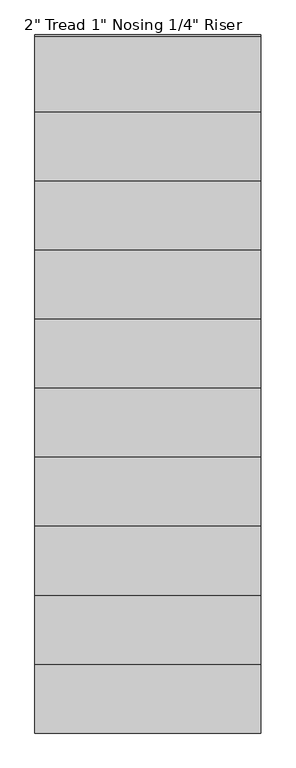
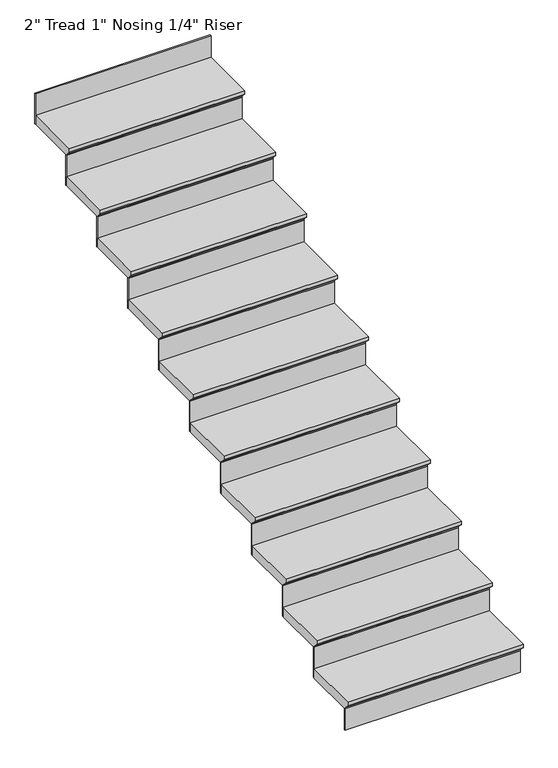
"""IFC4 building model written with IfcOpenShell, lengths in millimetres: stair flight geometry."""

from ifc_helpers import new_model, si_unit, origin, place, context, project, spatial, faceted_brep, source, transform, mapped, element, save


def stair_flight_5407f273(model_context):
    return source(origin(), model_context, "Body", "Brep", [
        faceted_brep([(-1200.9932736, 3353.09939, 150.2833333), (-1200.9932736, 3353.09939, 169.3333333), (-2115.3932736, 3353.09939, 169.3333333), (-2115.3932736, 3353.09939, 150.2833333), (-1200.9932736, 3378.49939, 124.8833333), (-2115.3932736, 3378.49939, 124.8833333), (-1200.9932736, 3657.89939, 169.3333333), (-2115.3932736, 3657.89939, 169.3333333), (-2115.3932736, 3378.49939, 118.5333333), (-2115.3932736, 3657.89939, 118.5333333), (-1200.9932736, 3657.89939, 118.5333333), (-1200.9932736, 3378.49939, 118.5333333)], [[[0, 1, 2, 3]], [[4, 0, 3, 5]], [[2, 1, 6, 7]], [[8, 9, 10, 11]], [[2, 7, 9, 8, 5, 3]], [[8, 11, 4, 5]], [[6, 1, 0, 4, 11, 10]], [[7, 6, 10, 9]]]),
        faceted_brep([(-1200.9932736, 3378.49939, 118.5333333), (-1200.9932736, 3378.49939, 0.0), (-1200.9932736, 3384.84939, 0.0), (-1200.9932736, 3384.84939, 118.5333333), (-2115.3932736, 3378.49939, 118.5333333), (-2115.3932736, 3384.84939, 118.5333333), (-2115.3932736, 3384.84939, 0.0), (-2115.3932736, 3378.49939, 0.0)], [[[0, 1, 2, 3]], [[4, 5, 6, 7]], [[1, 0, 4, 7]], [[2, 1, 7, 6]], [[3, 2, 6, 5]], [[0, 3, 5, 4]]]),
        faceted_brep([(-1200.9932736, 3657.89939, 287.8666667), (-1200.9932736, 3657.89939, 118.5333333), (-1200.9932736, 3664.24939, 118.5333333), (-1200.9932736, 3664.24939, 287.8666667), (-2115.3932736, 3657.89939, 287.8666667), (-2115.3932736, 3664.24939, 287.8666667), (-2115.3932736, 3664.24939, 118.5333333), (-2115.3932736, 3657.89939, 118.5333333)], [[[0, 1, 2, 3]], [[4, 5, 6, 7]], [[1, 0, 4, 7]], [[2, 1, 7, 6]], [[3, 2, 6, 5]], [[0, 3, 5, 4]]]),
        faceted_brep([(-2115.3932736, 3632.49939, 338.6666667), (-1200.9932736, 3632.49939, 338.6666667), (-1200.9932736, 3937.29939, 338.6666667), (-2115.3932736, 3937.29939, 338.6666667), (-2115.3932736, 3657.89939, 287.8666667), (-2115.3932736, 3937.29939, 287.8666667), (-1200.9932736, 3937.29939, 287.8666667), (-1200.9932736, 3657.89939, 287.8666667), (-2115.3932736, 3657.89939, 294.2166667), (-2115.3932736, 3632.49939, 319.6166667), (-1200.9932736, 3657.89939, 294.2166667), (-1200.9932736, 3632.49939, 319.6166667)], [[[0, 1, 2, 3]], [[4, 5, 6, 7]], [[0, 3, 5, 4, 8, 9]], [[4, 7, 10, 8]], [[2, 1, 11, 10, 7, 6]], [[3, 2, 6, 5]], [[11, 1, 0, 9]], [[10, 11, 9, 8]]]),
        faceted_brep([(-1200.9932736, 3937.29939, 457.2), (-1200.9932736, 3937.29939, 287.8666667), (-1200.9932736, 3943.64939, 287.8666667), (-1200.9932736, 3943.64939, 457.2), (-2115.3932736, 3937.29939, 457.2), (-2115.3932736, 3943.64939, 457.2), (-2115.3932736, 3943.64939, 287.8666667), (-2115.3932736, 3937.29939, 287.8666667)], [[[0, 1, 2, 3]], [[4, 5, 6, 7]], [[1, 0, 4, 7]], [[2, 1, 7, 6]], [[3, 2, 6, 5]], [[0, 3, 5, 4]]]),
        faceted_brep([(-2115.3932736, 3911.89939, 508.0), (-1200.9932736, 3911.89939, 508.0), (-1200.9932736, 4216.69939, 508.0), (-2115.3932736, 4216.69939, 508.0), (-2115.3932736, 3937.29939, 457.2), (-2115.3932736, 4216.69939, 457.2), (-1200.9932736, 4216.69939, 457.2), (-1200.9932736, 3937.29939, 457.2), (-2115.3932736, 3937.29939, 463.55), (-2115.3932736, 3911.89939, 488.95), (-1200.9932736, 3937.29939, 463.55), (-1200.9932736, 3911.89939, 488.95)], [[[0, 1, 2, 3]], [[4, 5, 6, 7]], [[0, 3, 5, 4, 8, 9]], [[4, 7, 10, 8]], [[2, 1, 11, 10, 7, 6]], [[3, 2, 6, 5]], [[11, 1, 0, 9]], [[10, 11, 9, 8]]]),
        faceted_brep([(-1200.9932736, 4216.69939, 626.5333333), (-1200.9932736, 4216.69939, 457.2), (-1200.9932736, 4223.04939, 457.2), (-1200.9932736, 4223.04939, 626.5333333), (-2115.3932736, 4216.69939, 626.5333333), (-2115.3932736, 4223.04939, 626.5333333), (-2115.3932736, 4223.04939, 457.2), (-2115.3932736, 4216.69939, 457.2)], [[[0, 1, 2, 3]], [[4, 5, 6, 7]], [[1, 0, 4, 7]], [[2, 1, 7, 6]], [[3, 2, 6, 5]], [[0, 3, 5, 4]]]),
        faceted_brep([(-2115.3932736, 4191.29939, 677.3333333), (-1200.9932736, 4191.29939, 677.3333333), (-1200.9932736, 4496.09939, 677.3333333), (-2115.3932736, 4496.09939, 677.3333333), (-2115.3932736, 4216.69939, 626.5333333), (-2115.3932736, 4496.09939, 626.5333333), (-1200.9932736, 4496.09939, 626.5333333), (-1200.9932736, 4216.69939, 626.5333333), (-2115.3932736, 4216.69939, 632.8833333), (-2115.3932736, 4191.29939, 658.2833333), (-1200.9932736, 4216.69939, 632.8833333), (-1200.9932736, 4191.29939, 658.2833333)], [[[0, 1, 2, 3]], [[4, 5, 6, 7]], [[0, 3, 5, 4, 8, 9]], [[4, 7, 10, 8]], [[2, 1, 11, 10, 7, 6]], [[3, 2, 6, 5]], [[11, 1, 0, 9]], [[10, 11, 9, 8]]]),
        faceted_brep([(-1200.9932736, 4496.09939, 795.8666667), (-1200.9932736, 4496.09939, 626.5333333), (-1200.9932736, 4502.44939, 626.5333333), (-1200.9932736, 4502.44939, 795.8666667), (-2115.3932736, 4496.09939, 795.8666667), (-2115.3932736, 4502.44939, 795.8666667), (-2115.3932736, 4502.44939, 626.5333333), (-2115.3932736, 4496.09939, 626.5333333)], [[[0, 1, 2, 3]], [[4, 5, 6, 7]], [[1, 0, 4, 7]], [[2, 1, 7, 6]], [[3, 2, 6, 5]], [[0, 3, 5, 4]]]),
        faceted_brep([(-2115.3932736, 4470.69939, 846.6666667), (-1200.9932736, 4470.69939, 846.6666667), (-1200.9932736, 4775.49939, 846.6666667), (-2115.3932736, 4775.49939, 846.6666667), (-2115.3932736, 4496.09939, 795.8666667), (-2115.3932736, 4775.49939, 795.8666667), (-1200.9932736, 4775.49939, 795.8666667), (-1200.9932736, 4496.09939, 795.8666667), (-2115.3932736, 4496.09939, 802.2166667), (-2115.3932736, 4470.69939, 827.6166667), (-1200.9932736, 4496.09939, 802.2166667), (-1200.9932736, 4470.69939, 827.6166667)], [[[0, 1, 2, 3]], [[4, 5, 6, 7]], [[0, 3, 5, 4, 8, 9]], [[4, 7, 10, 8]], [[2, 1, 11, 10, 7, 6]], [[3, 2, 6, 5]], [[11, 1, 0, 9]], [[10, 11, 9, 8]]]),
        faceted_brep([(-1200.9932736, 4775.49939, 965.2), (-1200.9932736, 4775.49939, 795.8666667), (-1200.9932736, 4781.84939, 795.8666667), (-1200.9932736, 4781.84939, 965.2), (-2115.3932736, 4775.49939, 965.2), (-2115.3932736, 4781.84939, 965.2), (-2115.3932736, 4781.84939, 795.8666667), (-2115.3932736, 4775.49939, 795.8666667)], [[[0, 1, 2, 3]], [[4, 5, 6, 7]], [[1, 0, 4, 7]], [[2, 1, 7, 6]], [[3, 2, 6, 5]], [[0, 3, 5, 4]]]),
        faceted_brep([(-2115.3932736, 4750.09939, 1016.0), (-1200.9932736, 4750.09939, 1016.0), (-1200.9932736, 5054.89939, 1016.0), (-2115.3932736, 5054.89939, 1016.0), (-2115.3932736, 4775.49939, 965.2), (-2115.3932736, 5054.89939, 965.2), (-1200.9932736, 5054.89939, 965.2), (-1200.9932736, 4775.49939, 965.2), (-2115.3932736, 4775.49939, 971.55), (-2115.3932736, 4750.09939, 996.95), (-1200.9932736, 4775.49939, 971.55), (-1200.9932736, 4750.09939, 996.95)], [[[0, 1, 2, 3]], [[4, 5, 6, 7]], [[0, 3, 5, 4, 8, 9]], [[4, 7, 10, 8]], [[2, 1, 11, 10, 7, 6]], [[3, 2, 6, 5]], [[11, 1, 0, 9]], [[10, 11, 9, 8]]]),
        faceted_brep([(-1200.9932736, 5054.89939, 1134.5333333), (-1200.9932736, 5054.89939, 965.2), (-1200.9932736, 5061.24939, 965.2), (-1200.9932736, 5061.24939, 1134.5333333), (-2115.3932736, 5054.89939, 1134.5333333), (-2115.3932736, 5061.24939, 1134.5333333), (-2115.3932736, 5061.24939, 965.2), (-2115.3932736, 5054.89939, 965.2)], [[[0, 1, 2, 3]], [[4, 5, 6, 7]], [[1, 0, 4, 7]], [[2, 1, 7, 6]], [[3, 2, 6, 5]], [[0, 3, 5, 4]]]),
        faceted_brep([(-2115.3932736, 5029.49939, 1185.3333333), (-1200.9932736, 5029.49939, 1185.3333333), (-1200.9932736, 5334.29939, 1185.3333333), (-2115.3932736, 5334.29939, 1185.3333333), (-2115.3932736, 5054.89939, 1134.5333333), (-2115.3932736, 5334.29939, 1134.5333333), (-1200.9932736, 5334.29939, 1134.5333333), (-1200.9932736, 5054.89939, 1134.5333333), (-2115.3932736, 5054.89939, 1140.8833333), (-2115.3932736, 5029.49939, 1166.2833333), (-1200.9932736, 5054.89939, 1140.8833333), (-1200.9932736, 5029.49939, 1166.2833333)], [[[0, 1, 2, 3]], [[4, 5, 6, 7]], [[0, 3, 5, 4, 8, 9]], [[4, 7, 10, 8]], [[2, 1, 11, 10, 7, 6]], [[3, 2, 6, 5]], [[11, 1, 0, 9]], [[10, 11, 9, 8]]]),
        faceted_brep([(-1200.9932736, 5334.29939, 1303.8666667), (-1200.9932736, 5334.29939, 1134.5333333), (-1200.9932736, 5340.64939, 1134.5333333), (-1200.9932736, 5340.64939, 1303.8666667), (-2115.3932736, 5334.29939, 1303.8666667), (-2115.3932736, 5340.64939, 1303.8666667), (-2115.3932736, 5340.64939, 1134.5333333), (-2115.3932736, 5334.29939, 1134.5333333)], [[[0, 1, 2, 3]], [[4, 5, 6, 7]], [[1, 0, 4, 7]], [[2, 1, 7, 6]], [[3, 2, 6, 5]], [[0, 3, 5, 4]]]),
        faceted_brep([(-2115.3932736, 5308.89939, 1354.6666667), (-1200.9932736, 5308.89939, 1354.6666667), (-1200.9932736, 5613.69939, 1354.6666667), (-2115.3932736, 5613.69939, 1354.6666667), (-2115.3932736, 5334.29939, 1303.8666667), (-2115.3932736, 5613.69939, 1303.8666667), (-1200.9932736, 5613.69939, 1303.8666667), (-1200.9932736, 5334.29939, 1303.8666667), (-2115.3932736, 5334.29939, 1310.2166667), (-2115.3932736, 5308.89939, 1335.6166667), (-1200.9932736, 5334.29939, 1310.2166667), (-1200.9932736, 5308.89939, 1335.6166667)], [[[0, 1, 2, 3]], [[4, 5, 6, 7]], [[0, 3, 5, 4, 8, 9]], [[4, 7, 10, 8]], [[2, 1, 11, 10, 7, 6]], [[3, 2, 6, 5]], [[11, 1, 0, 9]], [[10, 11, 9, 8]]]),
        faceted_brep([(-1200.9932736, 5613.69939, 1473.2), (-1200.9932736, 5613.69939, 1303.8666667), (-1200.9932736, 5620.04939, 1303.8666667), (-1200.9932736, 5620.04939, 1473.2), (-2115.3932736, 5613.69939, 1473.2), (-2115.3932736, 5620.04939, 1473.2), (-2115.3932736, 5620.04939, 1303.8666667), (-2115.3932736, 5613.69939, 1303.8666667)], [[[0, 1, 2, 3]], [[4, 5, 6, 7]], [[1, 0, 4, 7]], [[2, 1, 7, 6]], [[3, 2, 6, 5]], [[0, 3, 5, 4]]]),
        faceted_brep([(-2115.3932736, 5588.29939, 1524.0), (-1200.9932736, 5588.29939, 1524.0), (-1200.9932736, 5893.09939, 1524.0), (-2115.3932736, 5893.09939, 1524.0), (-2115.3932736, 5613.69939, 1473.2), (-2115.3932736, 5893.09939, 1473.2), (-1200.9932736, 5893.09939, 1473.2), (-1200.9932736, 5613.69939, 1473.2), (-2115.3932736, 5613.69939, 1479.55), (-2115.3932736, 5588.29939, 1504.95), (-1200.9932736, 5613.69939, 1479.55), (-1200.9932736, 5588.29939, 1504.95)], [[[0, 1, 2, 3]], [[4, 5, 6, 7]], [[0, 3, 5, 4, 8, 9]], [[4, 7, 10, 8]], [[2, 1, 11, 10, 7, 6]], [[3, 2, 6, 5]], [[11, 1, 0, 9]], [[10, 11, 9, 8]]]),
        faceted_brep([(-1200.9932736, 6172.49939, 1811.8666667), (-1200.9932736, 6172.49939, 1642.5333333), (-1200.9932736, 6178.84939, 1642.5333333), (-1200.9932736, 6178.84939, 1811.8666667), (-2115.3932736, 6172.49939, 1811.8666667), (-2115.3932736, 6178.84939, 1811.8666667), (-2115.3932736, 6178.84939, 1642.5333333), (-2115.3932736, 6172.49939, 1642.5333333)], [[[0, 1, 2, 3]], [[4, 5, 6, 7]], [[1, 0, 4, 7]], [[2, 1, 7, 6]], [[3, 2, 6, 5]], [[0, 3, 5, 4]]]),
        faceted_brep([(-1200.9932736, 5893.09939, 1642.5333333), (-1200.9932736, 5893.09939, 1473.2), (-1200.9932736, 5899.44939, 1473.2), (-1200.9932736, 5899.44939, 1642.5333333), (-2115.3932736, 5893.09939, 1642.5333333), (-2115.3932736, 5899.44939, 1642.5333333), (-2115.3932736, 5899.44939, 1473.2), (-2115.3932736, 5893.09939, 1473.2)], [[[0, 1, 2, 3]], [[4, 5, 6, 7]], [[1, 0, 4, 7]], [[2, 1, 7, 6]], [[3, 2, 6, 5]], [[0, 3, 5, 4]]]),
        faceted_brep([(-2115.3932736, 5867.69939, 1693.3333333), (-1200.9932736, 5867.69939, 1693.3333333), (-1200.9932736, 6147.09939, 1693.3333333), (-1200.9932736, 6172.49939, 1693.3333333), (-2115.3932736, 6172.49939, 1693.3333333), (-2115.3932736, 5893.09939, 1642.5333333), (-2115.3932736, 6172.49939, 1642.5333333), (-1200.9932736, 6172.49939, 1642.5333333), (-1200.9932736, 6147.09939, 1642.5333333), (-1200.9932736, 5893.09939, 1642.5333333), (-2115.3932736, 5893.09939, 1648.8833333), (-2115.3932736, 5867.69939, 1674.2833333), (-1200.9932736, 5893.09939, 1648.8833333), (-1200.9932736, 5867.69939, 1674.2833333)], [[[0, 1, 2, 3, 4]], [[5, 6, 7, 8, 9]], [[0, 4, 6, 5, 10, 11]], [[5, 9, 12, 10]], [[2, 1, 13, 12, 9, 8]], [[3, 2, 8, 7]], [[4, 3, 7, 6]], [[13, 1, 0, 11]], [[12, 13, 11, 10]]]),
    ])


if __name__ == "__main__":
    model = new_model("IFC4")
    model_context = context("Model", 3, world=origin())
    ifc_project = project(units=[si_unit("LENGTHUNIT", "METRE", prefix="MILLI")], contexts=[model_context])
    site = spatial("IfcSite", under=ifc_project)
    building = spatial("IfcBuilding", under=site)
    placement = place(None, origin())
    stair_flight_shape = stair_flight_5407f273(model_context)
    element("IfcStairFlight", 1, ObjectType="2\" Tread 1\" Nosing 1/4\" Riser", at=placement, inside=building, context=model_context, shape_type="MappedRepresentation", body=[
        mapped(stair_flight_shape, transform((0.0, 0.0, 0.0), x_axis=(1.0, 0.0, 0.0), y_axis=(0.0, 1.0, 0.0), z_axis=(0.0, 0.0, 1.0))),
    ])
    save(model, "model.ifc")
